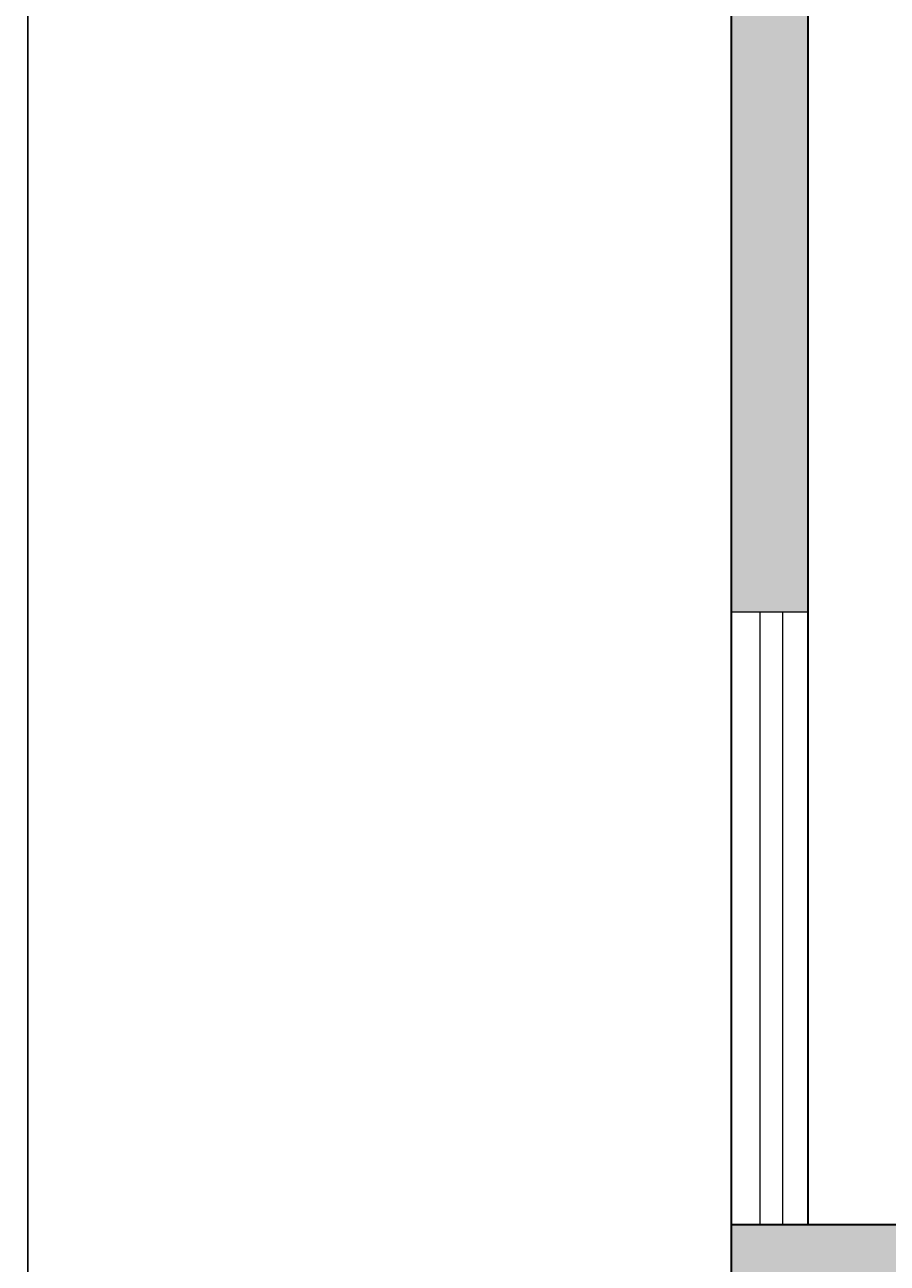
# Model space of a CAD drawing. Units: inches. Extents: x 192 to 1361, y -1362 to 367.
# Tile 3 of 23: x 192 to 293, y -761 to -616. Entities that reach past the tile are written whole.
import ezdxf

# ---------------------------------------------------------------- set-up
doc = ezdxf.new("R2010")
doc.units = ezdxf.units.IN
doc.header["$MEASUREMENT"] = 0
for name, color, linetype, lineweight in [('A-ANNO-DIMS', 2, 'Continuous', 18), ('A-WALL-PATT', 250, 'Continuous', 13), ('walls', 7, 'Continuous', 35), ('windows', 4, 'Continuous', 18)]:
    doc.layers.add(name, color=color, linetype=linetype, lineweight=lineweight)
doc.styles.get("Standard").update_dxf_attribs({"font": 'arial.ttf'})
doc.dimstyles.get("Standard").update_dxf_attribs({"dimtxt": 0.18, "dimasz": 0.18, "dimexe": 0.18, "dimexo": 0.0625, "dimgap": 0.09, "dimtad": 0, "dimtih": 1, "dimtoh": 1, "dimzin": 0, "dimdsep": 46, "dimlunit": 3, "dimtxsty": 'Standard', "dimcen": 0.09, "dimadec": 0, "dimazin": 0, "dimtfac": 1, "dimtofl": 0, "dimtmove": 0, "dimatfit": 3, "dimfxl": 1, "dimtolj": 1, "dimtzin": 0, "dimarcsym": 0})

# ---------------------------------------------------------------- blocks, each defined once
blk = doc.blocks.new('*D48')
at = {"layer": 'A-ANNO-DIMS', "color": 0, "lineweight": -2, "transparency": 16777216}
for p, q in [((325.63, 258.53), (192.16, 258.53)), ((192.34, 258.35), (192.34, -429.22)), ((192.34, -1117.14), (192.34, -429.58)), ((395.21, -1117.32), (192.16, -1117.32))]:
    blk.add_line(p, q, dxfattribs=at)
at = {"layer": 'A-ANNO-DIMS', "color": 0, "transparency": 16777216}
for points in [[(192.31, 258.35), (192.37, 258.35), (192.34, 258.53)], [(192.31, -1117.14), (192.37, -1117.14), (192.34, -1117.32)]]:
    blk.add_solid(points, dxfattribs=at)
at = {"layer": 'Defpoints', "color": 0, "transparency": 16777216}
for p in [(325.7, 258.53), (192.34, -1117.32), (395.28, -1117.32)]:
    blk.add_point(p, dxfattribs=at)
at = {"layer": 'A-ANNO-DIMS', "color": 0, "transparency": 16777216, "insert": (192.34, -429.4), "char_height": 0.18, "attachment_point": 5}
blk.add_mtext('\\A1;1375.9', dxfattribs=at)

msp = doc.modelspace()

# ---------------------------------------------------------------- hatches: boundary and pattern name
at = {"layer": 'A-WALL-PATT'}
h = msp.add_hatch(color=256, dxfattribs=at)
h.dxf.hatch_style = 1
h.paths.add_polyline_path([(309.5452, 191.102), (300.5452, 191.102), (300.5452, -126.898), (309.5452, -126.898), (309.5452, -117.898)])
h.paths.add_polyline_path([(420.798, 191.102), (337.3229, 191.102), (337.3229, 182.102), (420.798, 182.102)])
h.paths.add_polyline_path([(518.5452, 182.102), (625.4022, 182.102), (625.4022, 191.102), (509.5452, 191.102), (509.5452, 114.3262), (518.5452, 114.3262)])
h.paths.add_polyline_path([(842.5452, 191.102), (763.4438, 191.102), (763.4438, 182.102), (833.5452, 182.102), (833.5452, 161.1615), (836.8088, 161.1615), (842.5452, 161.1615)])
h.paths.add_polyline_path([(842.5452, -16.5675), (833.5452, -16.5675), (833.5452, -60.4996), (784.8041, -60.4996), (784.8041, -354.6796), (793.8041, -354.6796), (793.8041, -69.4996), (1094.1252, -69.4996), (1094.1252, -60.4996), (842.5452, -60.4996)])
h.paths.add_polyline_path([(518.5452, 36.602), (509.5452, 36.602), (509.5452, -117.898), (420.2204, -117.898), (420.2204, -126.898), (518.5452, -126.898)])
h.paths.add_polyline_path([(474.8041, -377.0384), (465.8041, -377.0384), (465.8041, -381.5384), (465.8041, -450.898), (537.5717, -450.898), (537.5717, -441.898), (474.8041, -441.898)])
h.paths.add_polyline_path([(1162.8041, -380.6763), (1204.3001, -380.6763), (1204.3001, -375.6763), (1195.1471, -375.6763), (1153.8041, -375.6763), (1153.8041, -448.4996), (856.5691, -448.4996), (856.5691, -457.4996), (1162.8041, -457.4996)])
h.paths.add_polyline_path([(1162.8041, -525.128), (1153.8041, -525.128), (1153.8041, -597.4996), (1162.8041, -597.4996)], flags=17)
h.paths.add_polyline_path([(1162.8041, -60.4996), (1153.8041, -60.4996), (1153.8041, -69.4996), (1153.8041, -177.4733), (1205.8889, -177.4733), (1205.8889, -172.4733), (1162.8041, -172.4733)])
h.paths.add_polyline_path([(980.5799, -525.686), (971.5799, -525.686), (971.5799, -597.4996), (980.5799, -597.4996)], flags=17)
h.paths.add_polyline_path([(856.5691, -448.4996), (798.7542, -448.4996), (784.8041, -448.4996), (784.8041, -457.4996), (847.5691, -457.4996), (847.5691, -597.4996), (784.8041, -597.4996), (784.8041, -606.4996), (1273.5658, -606.4996), (1273.5658, -597.4996), (856.5691, -597.4996)])
h.paths.add_polyline_path([(1273.5658, -773.892), (1099.8366, -773.892), (1099.8366, -851.9362), (1108.8366, -851.9362), (1108.8366, -782.892), (1273.5658, -782.892)])
h.paths.add_polyline_path([(1108.8366, -982.9214), (1099.8366, -982.9214), (1099.8366, -1067.6246), (1037.7563, -1067.6246), (1037.7563, -1076.6246), (1108.8366, -1076.6246)])
h.paths.add_polyline_path([(835.078, -1067.6246), (758.8458, -1067.6246), (758.8458, -940.2324), (749.8458, -940.2324), (749.8458, -963.172), (749.8458, -970.4644), (749.8458, -1076.6246), (835.078, -1076.6246)])
h.paths.add_polyline_path([(450.307, -1066.9838), (441.307, -1066.9838), (441.307, -1076.6246), (450.307, -1076.6246)])
h.paths.add_polyline_path([(492.8925, -756.4415), (274.8925, -756.4415), (274.8925, -765.4415), (492.8925, -765.4415)])
h.paths.add_polyline_path([(283.8925, -835.2244), (274.8925, -835.2244), (274.8925, -914.4415), (492.8925, -914.4415), (492.8925, -839.9415), (483.8925, -839.9415), (483.8925, -905.4415), (283.8925, -905.4415)])
h.paths.add_polyline_path([(283.8925, -441.898), (283.8925, -375.4296), (281.6021, -375.4296), (281.6021, -399.4121), (274.8925, -399.4121), (274.8925, -441.898), (274.8925, -684.5089), (283.8925, -684.5089)])

# ---------------------------------------------------------------- linework, layer by layer
at = {"layer": 'walls'}
for p, q in [((274.8925, -441.898), (274.8925, -914.4415)), ((283.8925, -441.898), (283.8925, -756.4415)), ((492.8925, -756.4415), (274.8925, -756.4415))]:
    msp.add_line(p, q, dxfattribs=at)
at = {"layer": 'windows'}
for p, q in [((274.8925, -684.5089), (283.8925, -684.5089)), ((278.2403, -684.5089), (278.2403, -756.4415)), ((280.9699, -756.4415), (280.9699, -684.5089))]:
    msp.add_line(p, q, dxfattribs=at)

# ---------------------------------------------------------------- dimensions: what is measured, and where the dimension line sits
at = {"layer": 'A-ANNO-DIMS'}
dim = msp.add_linear_dim(base=(192.3425, -1117.3227), p1=(325.6957, 258.5286), p2=(395.2768, -1117.3227), angle=90, dimstyle='Standard', override={"dimdec": 1, "dimlfac": 1, "dimrnd": 0, "dimzin": 0, "dimdsep": 46, "dimlunit": 2}, dxfattribs=at)
dim.commit()
dim.dimension.update_dxf_attribs({"geometry": '*D48', "text_midpoint": (192.3425, -429.3971)})

doc.saveas('drawing.dxf')
